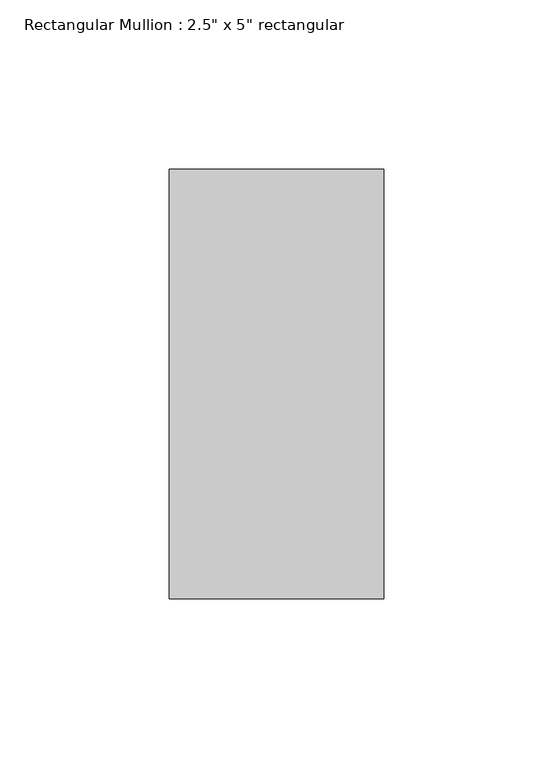
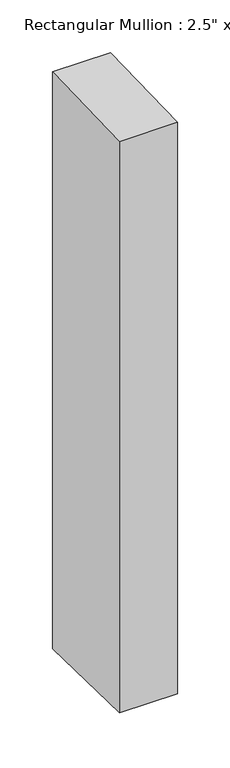
"""IFC4 building model written with IfcOpenShell, lengths in millimetres: member geometry."""

from ifc_helpers import new_model, si_unit, frame, origin, place, context, project, spatial, polyline, outline, extrude, source, transform, mapped, element, save


def member_1aee267e(model_context):
    return source(origin(), model_context, "Body", "SweptSolid", [
        extrude(outline(polyline([(-63.5, -1.9401005), (63.5, 1.9401005), (63.5, -666.6636602), (-63.5, -663.6152937), (-63.5, -1.9401005)])), frame((-63.5, 0.0, 0.0), z_axis=(1.0, 0.0, 0.0), x_axis=(0.0, 1.0, 0.0)), (0.0, 0.0, 1.0), 63.5),
    ])


if __name__ == "__main__":
    model = new_model("IFC4")
    model_context = context("Model", 3, world=origin())
    ifc_project = project(units=[si_unit("LENGTHUNIT", "METRE", prefix="MILLI")], contexts=[model_context])
    site = spatial("IfcSite", under=ifc_project)
    building = spatial("IfcBuilding", under=site)
    placement = place(None, origin())
    member_shape = member_1aee267e(model_context)
    element("IfcMember", 1, ObjectType="Rectangular Mullion : 2.5\" x 5\" rectangular", at=placement, inside=building, context=model_context, shape_type="MappedRepresentation", body=[
        mapped(member_shape, transform((0.0, 0.0, 0.0), x_axis=(1.0, 0.0, 0.0), y_axis=(0.0, 1.0, 0.0), z_axis=(0.0, 0.0, 1.0))),
    ])
    save(model, "model.ifc")

# Revit data of these elements
# Type "Rectangular Mullion : 2.5\" x 5\" rectangular"
#   built-in parameter 1007304 = 0.416667 (stored number, unit not read)
#   built-in parameter 1007301 = 0.104167 (stored number, unit not read)
#   built-in parameter 1007300 = 0.104167 (stored number, unit not read)
# Element 1 (IfcMember, "Rectangular Mullion : 2.5\" x 5\" rectangular")
#   Materials on its faces: "Aluminum"
# Materials
#   "Aluminum": class "Metal", colour RGB 247 247 247, transparency 0, Description = "Aluminum 6061", Cost = 0
